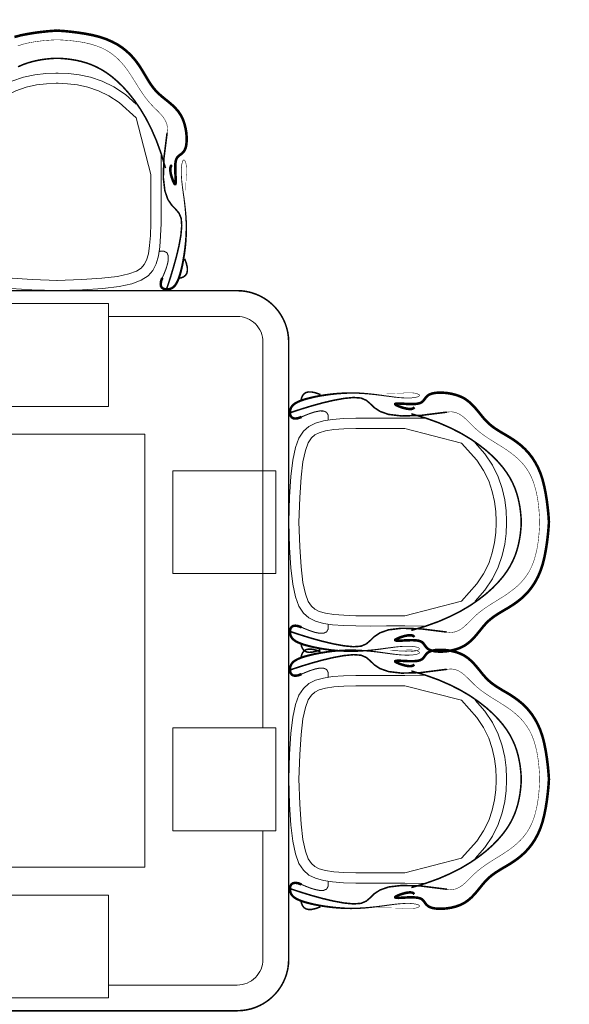
# Model space of a CAD drawing. Units: inches. Extents: x 513 to 1142, y 396 to 927.
# Tile 22 of 31: x 862 to 886, y 722 to 766. Entities that reach past the tile are written whole.
import ezdxf

# ---------------------------------------------------------------- set-up
doc = ezdxf.new("R2010")
doc.units = ezdxf.units.IN
doc.header["$MEASUREMENT"] = 0
doc.linetypes.add('DASHED', pattern=[0.75, 0.5, -0.25])
doc.layers.add('A-ANNO-DIMS', color=2, linetype='DASHED', lineweight=18)
doc.layers.add('furniture', color=92, linetype='Continuous', lineweight=18)
doc.styles.get("Standard").update_dxf_attribs({"font": 'arial.ttf'})
doc.dimstyles.get("Standard").update_dxf_attribs({"dimtxt": 4, "dimasz": 0.18, "dimexe": 0.18, "dimexo": 0.0625, "dimgap": 0.09, "dimtad": 0, "dimtih": 1, "dimtoh": 1, "dimdec": 0, "dimrnd": 6, "dimzin": 0, "dimdsep": 46, "dimlunit": 3, "dimtxsty": 'Standard', "dimcen": 0.09, "dimadec": 0, "dimazin": 0, "dimtfac": 1, "dimtdec": 0, "dimtofl": 0, "dimtmove": 0, "dimatfit": 3, "dimfxl": 1, "dimtolj": 1, "dimtzin": 0, "dimarcsym": 0})

# ---------------------------------------------------------------- blocks, each defined once
blk = doc.blocks.new('ОГ55_на6персон_стол1400х900')
at = {"const_width": 3}
blk.add_lwpolyline([(-600, 279.3), (600, 279.3, -0.414214), (700, 179.3), (700, -520.7, -0.414214), (600, -620.7), (-600, -620.7, -0.414214), (-700, -520.7), (-700, 179.3, -0.414214)], format="xyb", close=True, dxfattribs=at)
for points, const_width in [([(1193.2, -87.7), (1196.7, -101.2), (1199.4, -115.3), (1201.6, -129.2), (1203.2, -142.1), (1204.4, -153.5), (1205.1, -162.5), (1205.5, -168.5), (1205.7, -170.7)], 5), ([(1135.3, -94.9), (1139.6, -104.7), (1143, -114.3), (1145.6, -123.7), (1147.7, -132.7), (1149.2, -141.4), (1150.3, -149.3), (1151, -156.4), (1151.5, -162.3), (1151.7, -166.8), (1151.8, -169.6), (1151.8, -170.7)], 3), ([(1175.9, -94), (1179.3, -105.1), (1182.2, -117.4), (1184.5, -130.9), (1186.2, -145.8), (1187.4, -162.1), (1187.8, -170.7)], 1), ([(944.1, -394.1), (942.1, -391.9), (938.9, -390.8), (934.9, -390.6), (930.3, -391.1), (925.5, -392), (920.8, -393.4), (916.4, -394.9), (912.7, -396.3), (909.9, -397.6), (908, -398.7), (907.1, -399.6), (907.1, -400.3), (908, -400.8), (909.8, -401.1), (912.5, -401.2), (916.1, -401.2), (920.5, -401), (925.5, -400.7), (931, -400.4), (936.6, -400.2), (942.2, -400.3), (947.5, -400.6), (952.2, -401.3), (956.2, -402.5), (959.2, -404.2), (961.5, -406.4), (963.4, -408.8), (965.3, -411.4), (967.4, -414.1), (969.9, -416.5), (973.4, -418.7), (977.9, -420.5), (983.8, -421.8), (990.9, -422.4), (998.8, -422.4), (1007.3, -421.7), (1016.1, -420.3), (1024.9, -418), (1033.4, -415), (1041.3, -411), (1048.4, -406.2), (1054.8, -400.7), (1060.7, -394.6), (1066.3, -388.1), (1071.6, -381.6), (1076.9, -375), (1082.4, -368.7), (1088.1, -362.9), (1094.4, -357.6), (1101, -352.8), (1108, -348.2), (1115.2, -343.9), (1122.6, -339.5), (1130.1, -335), (1137.6, -330.2), (1145, -324.9), (1152.3, -319), (1159.4, -312.4), (1166.2, -305), (1172.7, -296.8), (1178.7, -287.6), (1184.1, -277.4), (1189, -266.1), (1193.2, -253.7), (1196.7, -240.1), (1199.4, -226.1), (1201.6, -212.2), (1203.2, -199.2), (1204.4, -187.9), (1205.1, -178.9), (1205.5, -172.9), (1205.7, -170.7)], 5), ([(938.3, -381.3), (966.1, -373), (991.4, -363.8), (1014.2, -353.9), (1034.8, -343.4), (1053.1, -332.5), (1069.4, -321.3), (1083.7, -310), (1096.1, -298.9), (1106.8, -287.9), (1116, -277.2), (1123.7, -266.7), (1130.1, -256.4), (1135.3, -246.4), (1139.6, -236.6), (1143, -227), (1145.6, -217.7), (1147.7, -208.6), (1149.2, -200), (1150.3, -192), (1151, -185), (1151.5, -179.1), (1151.7, -174.6), (1151.8, -171.7), (1151.8, -170.7)], 3), ([(1007.2, -384.5), (1015.9, -385.3), (1023.6, -384), (1030.7, -381.1), (1037.3, -376.9), (1043.5, -371.8), (1049.4, -366), (1055.3, -360), (1061.3, -354.1), (1067.5, -348.6), (1073.9, -343.4), (1080.6, -338.6), (1087.4, -334), (1094.3, -329.5), (1101.4, -325.1), (1108.5, -320.7), (1115.7, -316.1), (1122.9, -311.4), (1130, -306.5), (1137, -301.2), (1143.8, -295.4), (1150.3, -289.2), (1156.4, -282.3), (1162.1, -274.8), (1167.3, -266.5), (1171.9, -257.4), (1175.9, -247.3), (1179.3, -236.2), (1182.2, -224), (1184.5, -210.5), (1186.2, -195.6), (1187.4, -179.3), (1187.8, -170.7)], 1), ([(1007.2, -384.5), (956.2, -378.1), (919.4, -377.1), (894.1, -380.1), (877.3, -385.9), (866.4, -393.3), (858.5, -400.9), (850.8, -407.5), (840.7, -411.8), (826, -412.9), (807.4, -411.2), (786.6, -407.4), (765.2, -402.3), (744.5, -396.5), (726.1, -391), (711.6, -386.3), (702.6, -383.2)], 3), ([(724.9, -375.1), (732.7, -378.5), (741.6, -382), (751, -385), (760, -386.8), (767.8, -386.7), (773.6, -384.2), (776.8, -378.4), (776.4, -368.9)], 2), ([(761.7, -418.7), (752.5, -422), (744.8, -423.7), (738.5, -423.8), (733.5, -422.6), (729.7, -420.1), (726.9, -416.5), (725, -411.9), (723.8, -406.4)], 3), ([(-463.8, -927.9), (-457.4, -876.9), (-456.4, -840.1), (-459.4, -814.7), (-465.3, -798), (-472.6, -787), (-480.2, -779.2), (-486.8, -771.5), (-491.2, -761.4), (-492.3, -746.6), (-490.5, -728.1), (-486.7, -707.3), (-481.6, -685.8), (-475.9, -665.1), (-470.3, -646.8), (-465.6, -632.3), (-462.5, -623.2)], 3), ([(-36.2, -927.9), (-42.6, -876.9), (-43.6, -840.1), (-40.6, -814.7), (-34.7, -798), (-27.4, -787), (-19.8, -779.2), (-13.2, -771.5), (-8.8, -761.4), (-7.7, -746.6), (-9.5, -728.1), (-13.3, -707.3), (-18.4, -685.8), (-24.1, -665.1), (-29.7, -646.8), (-34.4, -632.3), (-37.5, -623.2)], 3), ([(36.2, -927.9), (42.6, -876.9), (43.6, -840.1), (40.6, -814.7), (34.7, -798), (27.4, -787), (19.8, -779.2), (13.2, -771.5), (8.8, -761.4), (7.7, -746.6), (9.5, -728.1), (13.3, -707.3), (18.4, -685.8), (24.1, -665.1), (29.7, -646.8), (34.4, -632.3), (37.5, -623.2)], 3), ([(463.8, -927.9), (457.4, -876.9), (456.4, -840.1), (459.4, -814.7), (465.3, -798), (472.6, -787), (480.2, -779.2), (486.8, -771.5), (491.2, -761.4), (492.3, -746.6), (490.5, -728.1), (486.7, -707.3), (481.6, -685.8), (475.9, -665.1), (470.3, -646.8), (465.6, -632.3), (462.5, -623.2)], 3), ([(-498, -682.4), (-501.3, -673.2), (-503, -665.5), (-503.1, -659.2), (-501.9, -654.2), (-499.4, -650.4), (-495.8, -647.6), (-491.2, -645.6), (-485.7, -644.5)], 3), ([(-454.5, -645.6), (-457.8, -653.4), (-461.3, -662.3), (-464.3, -671.7), (-466.1, -680.7), (-466, -688.5), (-463.5, -694.3), (-457.8, -697.5), (-448.2, -697.1)], 2), ([(-45.5, -645.6), (-42.2, -653.4), (-38.7, -662.3), (-35.7, -671.7), (-33.9, -680.7), (-34, -688.5), (-36.5, -694.3), (-42.2, -697.5), (-51.8, -697.1)], 2), ([(-2, -682.4), (1.3, -673.2), (3, -665.5), (3.1, -659.2), (1.9, -654.2), (-0.6, -650.4), (-4.2, -647.6), (-8.8, -645.6), (-14.3, -644.5)], 3), ([(2, -682.4), (-1.3, -673.2), (-3, -665.5), (-3.1, -659.2), (-1.9, -654.2), (0.6, -650.4), (4.2, -647.6), (8.8, -645.6), (14.3, -644.5)], 3), ([(45.5, -645.6), (42.2, -653.4), (38.7, -662.3), (35.7, -671.7), (33.9, -680.7), (34, -688.5), (36.5, -694.3), (42.2, -697.5), (51.8, -697.1)], 2), ([(454.5, -645.6), (457.8, -653.4), (461.3, -662.3), (464.3, -671.7), (466.1, -680.7), (466, -688.5), (463.5, -694.3), (457.8, -697.5), (448.2, -697.1)], 2), ([(498, -682.4), (501.3, -673.2), (503, -665.5), (503.1, -659.2), (501.9, -654.2), (499.4, -650.4), (495.8, -647.6), (491.2, -645.6), (485.7, -644.5)], 3), ([(-473.4, -864.8), (-471.2, -862.7), (-470.1, -859.6), (-469.9, -855.5), (-470.4, -851), (-471.4, -846.2), (-472.7, -841.5), (-474.2, -837.1), (-475.7, -833.4), (-477, -830.6), (-478, -828.7), (-478.9, -827.8), (-479.6, -827.7), (-480.1, -828.6), (-480.4, -830.5), (-480.6, -833.2), (-480.5, -836.7), (-480.3, -841.2), (-480, -846.2), (-479.7, -851.7), (-479.6, -857.3), (-479.6, -862.9), (-479.9, -868.2), (-480.6, -872.9), (-481.8, -876.8), (-483.5, -879.9), (-485.7, -882.2), (-488.2, -884.1), (-490.8, -886), (-493.4, -888), (-495.9, -890.6), (-498.1, -894), (-499.8, -898.6), (-501.1, -904.5), (-501.7, -911.6), (-501.7, -919.5), (-501, -928), (-499.6, -936.8), (-497.4, -945.6), (-494.3, -954.1), (-490.4, -962), (-485.5, -969.1), (-480, -975.5), (-473.9, -981.4), (-467.5, -986.9), (-460.9, -992.3), (-454.3, -997.6), (-448.1, -1003), (-442.2, -1008.8), (-436.9, -1015.1), (-432.1, -1021.7), (-427.6, -1028.7), (-423.2, -1035.9), (-418.9, -1043.3), (-414.4, -1050.8), (-409.5, -1058.3), (-404.2, -1065.7), (-398.3, -1073), (-391.7, -1080.1), (-384.3, -1086.9), (-376.1, -1093.3), (-366.9, -1099.3), (-356.7, -1104.8), (-345.4, -1109.7), (-333, -1113.9), (-319.5, -1117.3), (-305.4, -1120.1), (-291.5, -1122.3), (-278.6, -1123.9), (-267.2, -1125.1), (-258.2, -1125.8), (-252.2, -1126.2), (-250, -1126.3)], 5), ([(-26.6, -864.8), (-28.8, -862.7), (-29.9, -859.6), (-30.1, -855.5), (-29.6, -851), (-28.6, -846.2), (-27.3, -841.5), (-25.8, -837.1), (-24.3, -833.4), (-23, -830.6), (-22, -828.7), (-21.1, -827.8), (-20.4, -827.7), (-19.9, -828.6), (-19.6, -830.5), (-19.4, -833.2), (-19.5, -836.7), (-19.7, -841.2), (-20, -846.2), (-20.3, -851.7), (-20.4, -857.3), (-20.4, -862.9), (-20.1, -868.2), (-19.4, -872.9), (-18.2, -876.8), (-16.5, -879.9), (-14.3, -882.2), (-11.8, -884.1), (-9.2, -886), (-6.6, -888), (-4.1, -890.6), (-1.9, -894), (-0.2, -898.6), (1.1, -904.5), (1.7, -911.6), (1.7, -919.5), (1, -928), (-0.4, -936.8), (-2.6, -945.6), (-5.7, -954.1), (-9.6, -962), (-14.5, -969.1), (-20, -975.5), (-26.1, -981.4), (-32.5, -986.9), (-39.1, -992.3), (-45.7, -997.6), (-51.9, -1003), (-57.8, -1008.8), (-63.1, -1015.1), (-67.9, -1021.7), (-72.4, -1028.7), (-76.8, -1035.9), (-81.1, -1043.3), (-85.6, -1050.8), (-90.5, -1058.3), (-95.8, -1065.7), (-101.7, -1073), (-108.3, -1080.1), (-115.7, -1086.9), (-123.9, -1093.3), (-133.1, -1099.3), (-143.3, -1104.8), (-154.6, -1109.7), (-167, -1113.9), (-180.5, -1117.3), (-194.6, -1120.1), (-208.5, -1122.3), (-221.4, -1123.9), (-232.8, -1125.1), (-241.8, -1125.8), (-247.8, -1126.2), (-250, -1126.3)], 5), ([(26.6, -864.8), (28.8, -862.7), (29.9, -859.6), (30.1, -855.5), (29.6, -851), (28.6, -846.2), (27.3, -841.5), (25.8, -837.1), (24.3, -833.4), (23, -830.6), (22, -828.7), (21.1, -827.8), (20.4, -827.7), (19.9, -828.6), (19.6, -830.5), (19.4, -833.2), (19.5, -836.7), (19.7, -841.2), (20, -846.2), (20.3, -851.7), (20.4, -857.3), (20.4, -862.9), (20.1, -868.2), (19.4, -872.9), (18.2, -876.8), (16.5, -879.9), (14.3, -882.2), (11.8, -884.1), (9.2, -886), (6.6, -888), (4.1, -890.6), (1.9, -894), (0.2, -898.6), (-1.1, -904.5), (-1.7, -911.6), (-1.7, -919.5), (-1, -928), (0.4, -936.8), (2.6, -945.6), (5.7, -954.1), (9.6, -962), (14.5, -969.1), (20, -975.5), (26.1, -981.4), (32.5, -986.9), (39.1, -992.3), (45.7, -997.6), (51.9, -1003), (57.8, -1008.8), (63.1, -1015.1), (67.9, -1021.7), (72.4, -1028.7), (76.8, -1035.9), (81.1, -1043.3), (85.6, -1050.8), (90.5, -1058.3), (95.8, -1065.7), (101.7, -1073), (108.3, -1080.1), (115.7, -1086.9), (123.9, -1093.3), (133.1, -1099.3), (143.3, -1104.8), (154.6, -1109.7), (167, -1113.9), (180.5, -1117.3), (194.6, -1120.1), (208.5, -1122.3), (221.4, -1123.9), (232.8, -1125.1), (241.8, -1125.8), (247.8, -1126.2), (250, -1126.3)], 5), ([(473.4, -864.8), (471.2, -862.7), (470.1, -859.6), (469.9, -855.5), (470.4, -851), (471.4, -846.2), (472.7, -841.5), (474.2, -837.1), (475.7, -833.4), (477, -830.6), (478, -828.7), (478.9, -827.8), (479.6, -827.7), (480.1, -828.6), (480.4, -830.5), (480.6, -833.2), (480.5, -836.7), (480.3, -841.2), (480, -846.2), (479.7, -851.7), (479.6, -857.3), (479.6, -862.9), (479.9, -868.2), (480.6, -872.9), (481.8, -876.8), (483.5, -879.9), (485.7, -882.2), (488.2, -884.1), (490.8, -886), (493.4, -888), (495.9, -890.6), (498.1, -894), (499.8, -898.6), (501.1, -904.5), (501.7, -911.6), (501.7, -919.5), (501, -928), (499.6, -936.8), (497.4, -945.6), (494.3, -954.1), (490.4, -962), (485.5, -969.1), (480, -975.5), (473.9, -981.4), (467.5, -986.9), (460.9, -992.3), (454.3, -997.6), (448.1, -1003), (442.2, -1008.8), (436.9, -1015.1), (432.1, -1021.7), (427.6, -1028.7), (423.2, -1035.9), (418.9, -1043.3), (414.4, -1050.8), (409.5, -1058.3), (404.2, -1065.7), (398.3, -1073), (391.7, -1080.1), (384.3, -1086.9), (376.1, -1093.3), (366.9, -1099.3), (356.7, -1104.8), (345.4, -1109.7), (333, -1113.9), (319.5, -1117.3), (305.4, -1120.1), (291.5, -1122.3), (278.6, -1123.9), (267.2, -1125.1), (258.2, -1125.8), (252.2, -1126.2), (250, -1126.3)], 5), ([(-460.6, -859), (-452.3, -886.8), (-443.2, -912.1), (-433.2, -934.9), (-422.7, -955.5), (-411.8, -973.8), (-400.6, -990), (-389.4, -1004.3), (-378.2, -1016.8), (-367.2, -1027.5), (-356.5, -1036.7), (-346, -1044.4), (-335.8, -1050.8), (-325.7, -1056), (-315.9, -1060.3), (-306.4, -1063.6), (-297, -1066.3), (-287.9, -1068.3), (-279.3, -1069.9), (-271.3, -1071), (-264.3, -1071.7), (-258.4, -1072.2), (-253.9, -1072.4), (-251, -1072.5), (-250, -1072.5)], 3), ([(-39.4, -859), (-47.7, -886.8), (-56.8, -912.1), (-66.8, -934.9), (-77.3, -955.5), (-88.2, -973.8), (-99.4, -990), (-110.6, -1004.3), (-121.8, -1016.8), (-132.8, -1027.5), (-143.5, -1036.7), (-154, -1044.4), (-164.2, -1050.8), (-174.3, -1056), (-184.1, -1060.3), (-193.6, -1063.6), (-203, -1066.3), (-212.1, -1068.3), (-220.7, -1069.9), (-228.7, -1071), (-235.7, -1071.7), (-241.6, -1072.2), (-246.1, -1072.4), (-249, -1072.5), (-250, -1072.5)], 3), ([(39.4, -859), (47.7, -886.8), (56.8, -912.1), (66.8, -934.9), (77.3, -955.5), (88.2, -973.8), (99.4, -990), (110.6, -1004.3), (121.8, -1016.8), (132.8, -1027.5), (143.5, -1036.7), (154, -1044.4), (164.2, -1050.8), (174.3, -1056), (184.1, -1060.3), (193.6, -1063.6), (203, -1066.3), (212.1, -1068.3), (220.7, -1069.9), (228.7, -1071), (235.7, -1071.7), (241.6, -1072.2), (246.1, -1072.4), (249, -1072.5), (250, -1072.5)], 3), ([(460.6, -859), (452.3, -886.8), (443.2, -912.1), (433.2, -934.9), (422.7, -955.5), (411.8, -973.8), (400.6, -990), (389.4, -1004.3), (378.2, -1016.8), (367.2, -1027.5), (356.5, -1036.7), (346, -1044.4), (335.8, -1050.8), (325.7, -1056), (315.9, -1060.3), (306.4, -1063.6), (297, -1066.3), (287.9, -1068.3), (279.3, -1069.9), (271.3, -1071), (264.3, -1071.7), (258.4, -1072.2), (253.9, -1072.4), (251, -1072.5), (250, -1072.5)], 3), ([(-463.8, -927.9), (-464.6, -936.5), (-463.4, -944.3), (-460.5, -951.4), (-456.3, -958), (-451.1, -964.1), (-445.3, -970.1), (-439.3, -976), (-433.4, -982), (-427.9, -988.2), (-422.8, -994.6), (-417.9, -1001.3), (-413.3, -1008.1), (-408.8, -1015), (-404.4, -1022.1), (-400, -1029.2), (-395.5, -1036.4), (-390.8, -1043.6), (-385.8, -1050.7), (-380.5, -1057.7), (-374.7, -1064.5), (-368.5, -1071), (-361.7, -1077.1), (-354.1, -1082.8), (-345.9, -1088), (-336.7, -1092.6), (-326.7, -1096.6), (-315.5, -1100), (-303.3, -1102.9), (-289.8, -1105.2), (-274.9, -1106.9), (-258.6, -1108.1), (-250, -1108.4)], 1), ([(-36.2, -927.9), (-35.4, -936.5), (-36.6, -944.3), (-39.5, -951.4), (-43.7, -958), (-48.9, -964.1), (-54.7, -970.1), (-60.7, -976), (-66.6, -982), (-72.1, -988.2), (-77.2, -994.6), (-82.1, -1001.3), (-86.7, -1008.1), (-91.2, -1015), (-95.6, -1022.1), (-100, -1029.2), (-104.5, -1036.4), (-109.2, -1043.6), (-114.2, -1050.7), (-119.5, -1057.7), (-125.3, -1064.5), (-131.5, -1071), (-138.3, -1077.1), (-145.9, -1082.8), (-154.1, -1088), (-163.3, -1092.6), (-173.3, -1096.6), (-184.5, -1100), (-196.7, -1102.9), (-210.2, -1105.2), (-225.1, -1106.9), (-241.4, -1108.1), (-250, -1108.4)], 1), ([(36.2, -927.9), (35.4, -936.5), (36.6, -944.3), (39.5, -951.4), (43.7, -958), (48.9, -964.1), (54.7, -970.1), (60.7, -976), (66.6, -982), (72.1, -988.2), (77.2, -994.6), (82.1, -1001.3), (86.7, -1008.1), (91.2, -1015), (95.6, -1022.1), (100, -1029.2), (104.5, -1036.4), (109.2, -1043.6), (114.2, -1050.7), (119.5, -1057.7), (125.3, -1064.5), (131.5, -1071), (138.3, -1077.1), (145.9, -1082.8), (154.1, -1088), (163.3, -1092.6), (173.3, -1096.6), (184.5, -1100), (196.7, -1102.9), (210.2, -1105.2), (225.1, -1106.9), (241.4, -1108.1), (250, -1108.4)], 1), ([(463.8, -927.9), (464.6, -936.5), (463.4, -944.3), (460.5, -951.4), (456.3, -958), (451.1, -964.1), (445.3, -970.1), (439.3, -976), (433.4, -982), (427.9, -988.2), (422.8, -994.6), (417.9, -1001.3), (413.3, -1008.1), (408.8, -1015), (404.4, -1022.1), (400, -1029.2), (395.5, -1036.4), (390.8, -1043.6), (385.8, -1050.7), (380.5, -1057.7), (374.7, -1064.5), (368.5, -1071), (361.7, -1077.1), (354.1, -1082.8), (345.9, -1088), (336.7, -1092.6), (326.7, -1096.6), (315.5, -1100), (303.3, -1102.9), (289.8, -1105.2), (274.9, -1106.9), (258.6, -1108.1), (250, -1108.4)], 1)]:
    blk.add_lwpolyline(points, dxfattribs=dict(const_width=const_width))
for points in [[(966.1, 31.7), (925.8, 31.2), (889.9, 31.2), (858.2, 31.3), (830.4, 31.2), (806.3, 30.5), (785.4, 29), (767.4, 26.2), (752.2, 21.8), (739.4, 15.4), (728.7, 6.1), (720.1, -7.2), (713.2, -25.6), (708, -50.1), (704.2, -81.7), (701.6, -121.6), (700, -170.7)], [(1035.7, -17.1), (925.9, 11.2), (889.9, 11.2), (858.2, 11.3), (830.8, 11.2), (807.3, 10.5), (787.6, 9.1), (771.7, 6.6), (759.5, 3.1), (750.6, -1.3), (744, -7.1), (738, -16.3), (732.5, -31.2), (727.7, -53.4), (724.1, -83.6), (721.5, -122.5), (720, -171.3)], [(1035.7, -17.1), (1065.6, -50.4), (1078.8, -70.2), (1088.7, -90.5), (1095.5, -110.8), (1100, -130.9), (1102.3, -150.3), (1103.1, -168.6), (1103.1, -170.3)], [(1062.3, -16.7), (1081.4, -38.1), (1096.2, -60.3), (1107.2, -82.9), (1114.8, -105.5), (1119.7, -127.5), (1122.3, -148.6), (1123.1, -168.3), (1123.1, -170.7)], [(966.1, -373), (925.8, -372.6), (889.9, -372.6), (858.2, -372.7), (830.4, -372.6), (806.3, -371.9), (785.4, -370.3), (767.4, -367.5), (752.2, -363.2), (739.4, -356.8), (728.7, -347.5), (720.1, -334.1), (713.2, -315.8), (708, -291.3), (704.2, -259.6), (701.6, -219.8), (700, -170.7)], [(1035.7, -324.3), (925.9, -352.6), (889.9, -352.6), (858.2, -352.7), (830.8, -352.6), (807.3, -351.9), (787.6, -350.4), (771.7, -348), (759.5, -344.4), (750.6, -340), (744, -334.2), (738, -325.1), (732.5, -310.2), (727.7, -288), (724.1, -257.8), (721.5, -218.8), (720, -170)], [(1035.7, -324.3), (1065.6, -291), (1078.8, -271.1), (1088.7, -250.9), (1095.5, -230.5), (1100, -210.5), (1102.3, -191.1), (1103.1, -172.8), (1103.1, -171.1)], [(1062.3, -324.6), (1081.4, -303.3), (1096.2, -281.1), (1107.2, -258.5), (1114.8, -235.9), (1119.7, -213.8), (1122.3, -192.7), (1123.1, -173), (1123.1, -170.7)], [(-452.3, -886.8), (-451.9, -846.4), (-451.9, -810.6), (-452, -778.9), (-451.9, -751.1), (-451.2, -726.9), (-449.6, -706), (-446.8, -688.1), (-442.5, -672.9), (-436.1, -660), (-426.8, -649.4), (-413.5, -640.7), (-395.1, -633.9), (-370.6, -628.7), (-339, -624.8), (-299.1, -622.2), (-250, -620.7)], [(-47.7, -886.8), (-48.1, -846.4), (-48.1, -810.6), (-48, -778.9), (-48.1, -751.1), (-48.8, -726.9), (-50.4, -706), (-53.2, -688.1), (-57.5, -672.9), (-63.9, -660), (-73.2, -649.4), (-86.5, -640.7), (-104.9, -633.9), (-129.4, -628.7), (-161, -624.8), (-200.9, -622.2), (-250, -620.7)], [(47.7, -886.8), (48.1, -846.4), (48.1, -810.6), (48, -778.9), (48.1, -751.1), (48.8, -726.9), (50.4, -706), (53.2, -688.1), (57.5, -672.9), (63.9, -660), (73.2, -649.4), (86.5, -640.7), (104.9, -633.9), (129.4, -628.7), (161, -624.8), (200.9, -622.2), (250, -620.7)], [(452.3, -886.8), (451.9, -846.4), (451.9, -810.6), (452, -778.9), (451.9, -751.1), (451.2, -726.9), (449.6, -706), (446.8, -688.1), (442.5, -672.9), (436.1, -660), (426.8, -649.4), (413.5, -640.7), (395.1, -633.9), (370.6, -628.7), (339, -624.8), (299.1, -622.2), (250, -620.7)], [(-403.6, -956.4), (-431.9, -846.6), (-431.9, -810.5), (-432, -778.9), (-431.9, -751.4), (-431.2, -728), (-429.8, -708.3), (-427.3, -692.4), (-423.8, -680.1), (-419.4, -671.3), (-413.6, -664.7), (-404.4, -658.7), (-389.5, -653.1), (-367.3, -648.4), (-337.1, -644.8), (-298.1, -642.2), (-249.4, -640.7)], [(-96.4, -956.4), (-68.1, -846.6), (-68.1, -810.5), (-68, -778.9), (-68.1, -751.4), (-68.8, -728), (-70.2, -708.3), (-72.7, -692.4), (-76.2, -680.1), (-80.6, -671.3), (-86.4, -664.7), (-95.6, -658.7), (-110.5, -653.1), (-132.7, -648.4), (-162.9, -644.8), (-201.9, -642.2), (-250.6, -640.7)], [(96.4, -956.4), (68.1, -846.6), (68.1, -810.5), (68, -778.9), (68.1, -751.4), (68.8, -728), (70.2, -708.3), (72.7, -692.4), (76.2, -680.1), (80.6, -671.3), (86.4, -664.7), (95.6, -658.7), (110.5, -653.1), (132.7, -648.4), (162.9, -644.8), (201.9, -642.2), (250.6, -640.7)], [(403.6, -956.4), (431.9, -846.6), (431.9, -810.5), (432, -778.9), (431.9, -751.4), (431.2, -728), (429.8, -708.3), (427.3, -692.4), (423.8, -680.1), (419.4, -671.3), (413.6, -664.7), (404.4, -658.7), (389.5, -653.1), (367.3, -648.4), (337.1, -644.8), (298.1, -642.2), (249.4, -640.7)], [(-403.6, -956.4), (-370.3, -986.3), (-350.5, -999.5), (-330.2, -1009.3), (-309.8, -1016.2), (-289.8, -1020.6), (-270.4, -1023), (-252.1, -1023.8), (-250.4, -1023.8)], [(-96.4, -956.4), (-129.7, -986.3), (-149.5, -999.5), (-169.8, -1009.3), (-190.2, -1016.2), (-210.2, -1020.6), (-229.6, -1023), (-247.9, -1023.8), (-249.6, -1023.8)], [(96.4, -956.4), (129.7, -986.3), (149.5, -999.5), (169.8, -1009.3), (190.2, -1016.2), (210.2, -1020.6), (229.6, -1023), (247.9, -1023.8), (249.6, -1023.8)], [(403.6, -956.4), (370.3, -986.3), (350.5, -999.5), (330.2, -1009.3), (309.8, -1016.2), (289.8, -1020.6), (270.4, -1023), (252.1, -1023.8), (250.4, -1023.8)], [(-404, -983), (-382.6, -1002.1), (-360.4, -1016.9), (-337.8, -1027.9), (-315.2, -1035.5), (-293.1, -1040.4), (-272, -1043), (-252.3, -1043.8), (-250, -1043.8)], [(-96, -983), (-117.4, -1002.1), (-139.6, -1016.9), (-162.2, -1027.9), (-184.8, -1035.5), (-206.9, -1040.4), (-228, -1043), (-247.7, -1043.8), (-250, -1043.8)], [(96, -983), (117.4, -1002.1), (139.6, -1016.9), (162.2, -1027.9), (184.8, -1035.5), (206.9, -1040.4), (228, -1043), (247.7, -1043.8), (250, -1043.8)], [(404, -983), (382.6, -1002.1), (360.4, -1016.9), (337.8, -1027.9), (315.2, -1035.5), (293.1, -1040.4), (272, -1043), (252.3, -1043.8), (250, -1043.8)]]:
    blk.add_lwpolyline(points)
for points in [[(-420.7, -341.4), (420.7, -341.4), (420.7, 0), (-420.7, 0)], [(-675, -270.7), (-475, -270.7), (-475, -70.7), (-675, -70.7)], [(675, -270.7), (475, -270.7), (475, -70.7), (675, -70.7)], [(-150, -595.7), (-150, -395.7), (-350, -395.7), (-350, -595.7)], [(150, -595.7), (150, -395.7), (350, -395.7), (350, -595.7)]]:
    blk.add_lwpolyline(points, close=True)
for points, format in [([(-350, -570.7), (-600, -570.7, -0.414214), (-650, -520.7), (-650, -270.7)], "xyb"), ([(650, -270.7), (650, -520.7, -0.414214), (600, -570.7), (-150, -570.7)], "xyb"), ([(724.9, -375.1, 5, 4.91, 0), (718.1, -372.7, 4.91, 4.84, 0), (712.8, -372, 4.84, 4.78, 0), (708.7, -372.6, 4.78, 4.74, 0), (705.8, -374.3, 4.74, 4.7, 0), (703.9, -376.9, 4.7, 4.65, 0), (702.9, -380.1, 4.65, 4.61, 0), (702.5, -383.6, 4.61, 4.56, 0), (702.8, -387.1, 4.56, 4.52, 0), (703.5, -390.5, 4.52, 4.47, 0), (704.8, -393.6, 4.47, 4.43, 0), (706.7, -396.6, 4.43, 4.38, 0), (709.5, -399.3, 4.38, 4.32, 0), (713.2, -402, 4.32, 4.25, 0), (717.9, -404.5, 4.25, 4.17, 0), (723.8, -407, 4.17, 4.07, 0), (731, -409.4, 4.07, 3.95, 0), (739.6, -411.7, 3.95, 3.82, 0), (749.3, -414, 3.82, 3.68, 0), (760.1, -416, 3.68, 3.53, 0), (771.6, -417.9, 3.53, 3.37, 0), (783.7, -419.5, 3.37, 3.21, 0), (796.2, -420.7, 3.21, 3.05, 0), (808.8, -421.5, 3.05, 2.88, 0), (821.4, -421.8, 2.88, 2.72, 0), (833.8, -421.6, 2.72, 2.57, 0), (845.8, -420.9, 2.57, 2.41, 0), (857.4, -419.9, 2.41, 2.27, 0), (868.5, -418.7, 2.27, 2.13, 0), (879, -417.4, 2.13, 2, 0), (888.9, -416, 2, 1.88, 0), (898, -414.7, 1.88, 1.78, 0), (906.3, -413.7, 1.78, 1.68, 0), (913.7, -412.9, 1.68, 1.59, 0), (920.3, -412.4, 1.59, 1.52, 0), (926.1, -412.1, 1.52, 1.45, 0), (931.2, -412, 1.45, 1.4, 0), (935.6, -412.1, 1.4, 1.35, 0), (939.4, -412.3, 1.35, 1.3, 0), (942.6, -412.7, 1.3, 1.27, 0), (945.3, -413, 1.27, 1.24, 0), (947.6, -413.5, 1.24, 1.21, 0), (949.5, -413.9, 1.21, 1.19, 0), (951, -414.4, 1.19, 1.18, 0), (952.2, -414.9, 1.18, 1.16, 0), (953, -415.4, 1.16, 1.15, 0), (953.6, -416, 1.15, 1.14, 0), (953.9, -416.5, 1.14, 1.14, 0), (954, -417, 1.14, 1.13, 0), (953.9, -417.5, 1.13, 1.12, 0), (953.6, -418, 1.12, 1.12, 0), (953.2, -418.5, 1.12, 1.11, 0), (952.6, -418.9, 1.11, 1.09, 0), (951.8, -419.4, 1.09, 1.08, 0), (950.9, -419.8, 1.08, 1.07, 0), (949.8, -420.2, 1.07, 1.05, 0), (948.6, -420.6, 1.05, 1.03, 0), (947.2, -421, 1.03, 1.01, 0), (945.6, -421.3, 1.01, 0.986, 0), (943.8, -421.6, 0.986, 0.959, 0), (941.7, -421.8, 0.959, 0.926, 0), (939.2, -422, 0.926, 0.889, 0), (936.3, -422, 0.889, 0.846, 0), (933, -422, 0.846, 0.796, 0), (929.1, -422, 0.796, 0.738, 0), (924.7, -421.8, 0.738, 0.672, 0), (919.6, -421.5, 0.672, 0.595, 0), (913.7, -421.2, 0.595, 0.506, 0), (906.8, -421, 0.506, 0.404, 0), (898.9, -420.7, 0.404, 0.286, 0), (889.9, -420.6, 0.286, 0.152, 0), (879.5, -420.6, 0.152, 0, 0), (867.8, -420.7, 0, 0, 0)], "xyseb"), ([(-454.5, -645.6, 5, 4.91, 0), (-452, -638.8, 4.91, 4.84, 0), (-451.3, -633.5, 4.84, 4.78, 0), (-451.9, -629.4, 4.78, 4.74, 0), (-453.7, -626.5, 4.74, 4.7, 0), (-456.3, -624.6, 4.7, 4.65, 0), (-459.4, -623.5, 4.65, 4.61, 0), (-462.9, -623.2, 4.61, 4.56, 0), (-466.5, -623.5, 4.56, 4.52, 0), (-469.8, -624.2, 4.52, 4.47, 0), (-472.9, -625.5, 4.47, 4.43, 0), (-475.9, -627.4, 4.43, 4.38, 0), (-478.7, -630.2, 4.38, 4.32, 0), (-481.3, -633.9, 4.32, 4.25, 0), (-483.8, -638.6, 4.25, 4.17, 0), (-486.3, -644.5, 4.17, 4.07, 0), (-488.7, -651.7, 4.07, 3.95, 0), (-491, -660.3, 3.95, 3.82, 0), (-493.3, -670, 3.82, 3.68, 0), (-495.4, -680.8, 3.68, 3.53, 0), (-497.2, -692.3, 3.53, 3.37, 0), (-498.8, -704.4, 3.37, 3.21, 0), (-500, -716.9, 3.21, 3.05, 0), (-500.8, -729.5, 3.05, 2.88, 0), (-501.1, -742.1, 2.88, 2.72, 0), (-500.9, -754.5, 2.72, 2.57, 0), (-500.2, -766.5, 2.57, 2.41, 0), (-499.2, -778.1, 2.41, 2.27, 0), (-498, -789.2, 2.27, 2.13, 0), (-496.7, -799.7, 2.13, 2, 0), (-495.3, -809.6, 2, 1.88, 0), (-494.1, -818.7, 1.88, 1.78, 0), (-493, -827, 1.78, 1.68, 0), (-492.2, -834.4, 1.68, 1.59, 0), (-491.7, -841, 1.59, 1.52, 0), (-491.4, -846.8, 1.52, 1.45, 0), (-491.3, -851.9, 1.45, 1.4, 0), (-491.4, -856.3, 1.4, 1.35, 0), (-491.6, -860.1, 1.35, 1.3, 0), (-492, -863.3, 1.3, 1.27, 0), (-492.4, -866, 1.27, 1.24, 0), (-492.8, -868.3, 1.24, 1.21, 0), (-493.3, -870.2, 1.21, 1.19, 0), (-493.8, -871.7, 1.19, 1.18, 0), (-494.3, -872.9, 1.18, 1.16, 0), (-494.8, -873.7, 1.16, 1.15, 0), (-495.3, -874.3, 1.15, 1.14, 0), (-495.8, -874.6, 1.14, 1.14, 0), (-496.3, -874.7, 1.14, 1.13, 0), (-496.8, -874.6, 1.13, 1.12, 0), (-497.3, -874.3, 1.12, 1.12, 0), (-497.8, -873.9, 1.12, 1.11, 0), (-498.3, -873.3, 1.11, 1.09, 0), (-498.7, -872.5, 1.09, 1.08, 0), (-499.1, -871.6, 1.08, 1.07, 0), (-499.5, -870.5, 1.07, 1.05, 0), (-499.9, -869.2, 1.05, 1.03, 0), (-500.3, -867.9, 1.03, 1.01, 0), (-500.6, -866.3, 1.01, 0.986, 0), (-500.9, -864.5, 0.986, 0.959, 0), (-501.1, -862.4, 0.959, 0.926, 0), (-501.3, -859.9, 0.926, 0.889, 0), (-501.4, -857, 0.889, 0.846, 0), (-501.4, -853.7, 0.846, 0.796, 0), (-501.3, -849.8, 0.796, 0.738, 0), (-501.1, -845.4, 0.738, 0.672, 0), (-500.8, -840.3, 0.672, 0.595, 0), (-500.6, -834.3, 0.595, 0.506, 0), (-500.3, -827.5, 0.506, 0.404, 0), (-500.1, -819.6, 0.404, 0.286, 0), (-499.9, -810.5, 0.286, 0.152, 0), (-499.9, -800.2, 0.152, 0, 0), (-500, -788.5, 0, 0, 0)], "xyseb"), ([(-45.5, -645.6, 5, 4.91, 0), (-48, -638.8, 4.91, 4.84, 0), (-48.7, -633.5, 4.84, 4.78, 0), (-48.1, -629.4, 4.78, 4.74, 0), (-46.3, -626.5, 4.74, 4.7, 0), (-43.7, -624.6, 4.7, 4.65, 0), (-40.6, -623.5, 4.65, 4.61, 0), (-37.1, -623.2, 4.61, 4.56, 0), (-33.5, -623.5, 4.56, 4.52, 0), (-30.2, -624.2, 4.52, 4.47, 0), (-27.1, -625.5, 4.47, 4.43, 0), (-24.1, -627.4, 4.43, 4.38, 0), (-21.3, -630.2, 4.38, 4.32, 0), (-18.7, -633.9, 4.32, 4.25, 0), (-16.2, -638.6, 4.25, 4.17, 0), (-13.7, -644.5, 4.17, 4.07, 0), (-11.3, -651.7, 4.07, 3.95, 0), (-9, -660.3, 3.95, 3.82, 0), (-6.7, -670, 3.82, 3.68, 0), (-4.6, -680.8, 3.68, 3.53, 0), (-2.8, -692.3, 3.53, 3.37, 0), (-1.2, -704.4, 3.37, 3.21, 0), (0, -716.9, 3.21, 3.05, 0), (0.8, -729.5, 3.05, 2.88, 0), (1.1, -742.1, 2.88, 2.72, 0), (0.9, -754.5, 2.72, 2.57, 0), (0.2, -766.5, 2.57, 2.41, 0), (-0.8, -778.1, 2.41, 2.27, 0), (-2, -789.2, 2.27, 2.13, 0), (-3.3, -799.7, 2.13, 2, 0), (-4.7, -809.6, 2, 1.88, 0), (-5.9, -818.7, 1.88, 1.78, 0), (-7, -827, 1.78, 1.68, 0), (-7.8, -834.4, 1.68, 1.59, 0), (-8.3, -841, 1.59, 1.52, 0), (-8.6, -846.8, 1.52, 1.45, 0), (-8.7, -851.9, 1.45, 1.4, 0), (-8.6, -856.3, 1.4, 1.35, 0), (-8.4, -860.1, 1.35, 1.3, 0), (-8, -863.3, 1.3, 1.27, 0), (-7.6, -866, 1.27, 1.24, 0), (-7.2, -868.3, 1.24, 1.21, 0), (-6.7, -870.2, 1.21, 1.19, 0), (-6.2, -871.7, 1.19, 1.18, 0), (-5.7, -872.9, 1.18, 1.16, 0), (-5.2, -873.7, 1.16, 1.15, 0), (-4.7, -874.3, 1.15, 1.14, 0), (-4.2, -874.6, 1.14, 1.14, 0), (-3.7, -874.7, 1.14, 1.13, 0), (-3.2, -874.6, 1.13, 1.12, 0), (-2.7, -874.3, 1.12, 1.12, 0), (-2.2, -873.9, 1.12, 1.11, 0), (-1.7, -873.3, 1.11, 1.09, 0), (-1.3, -872.5, 1.09, 1.08, 0), (-0.9, -871.6, 1.08, 1.07, 0), (-0.5, -870.5, 1.07, 1.05, 0), (-0.1, -869.2, 1.05, 1.03, 0), (0.3, -867.9, 1.03, 1.01, 0), (0.6, -866.3, 1.01, 0.986, 0), (0.9, -864.5, 0.986, 0.959, 0), (1.1, -862.4, 0.959, 0.926, 0), (1.3, -859.9, 0.926, 0.889, 0), (1.4, -857, 0.889, 0.846, 0), (1.4, -853.7, 0.846, 0.796, 0), (1.3, -849.8, 0.796, 0.738, 0), (1.1, -845.4, 0.738, 0.672, 0), (0.8, -840.3, 0.672, 0.595, 0), (0.6, -834.3, 0.595, 0.506, 0), (0.3, -827.5, 0.506, 0.404, 0), (0.1, -819.6, 0.404, 0.286, 0), (-0.1, -810.5, 0.286, 0.152, 0), (-0.1, -800.2, 0.152, 0, 0), (0, -788.5, 0, 0, 0)], "xyseb"), ([(45.5, -645.6, 5, 4.91, 0), (48, -638.8, 4.91, 4.84, 0), (48.7, -633.5, 4.84, 4.78, 0), (48.1, -629.4, 4.78, 4.74, 0), (46.3, -626.5, 4.74, 4.7, 0), (43.7, -624.6, 4.7, 4.65, 0), (40.6, -623.5, 4.65, 4.61, 0), (37.1, -623.2, 4.61, 4.56, 0), (33.5, -623.5, 4.56, 4.52, 0), (30.2, -624.2, 4.52, 4.47, 0), (27.1, -625.5, 4.47, 4.43, 0), (24.1, -627.4, 4.43, 4.38, 0), (21.3, -630.2, 4.38, 4.32, 0), (18.7, -633.9, 4.32, 4.25, 0), (16.2, -638.6, 4.25, 4.17, 0), (13.7, -644.5, 4.17, 4.07, 0), (11.3, -651.7, 4.07, 3.95, 0), (9, -660.3, 3.95, 3.82, 0), (6.7, -670, 3.82, 3.68, 0), (4.6, -680.8, 3.68, 3.53, 0), (2.8, -692.3, 3.53, 3.37, 0), (1.2, -704.4, 3.37, 3.21, 0), (0, -716.9, 3.21, 3.05, 0), (-0.8, -729.5, 3.05, 2.88, 0), (-1.1, -742.1, 2.88, 2.72, 0), (-0.9, -754.5, 2.72, 2.57, 0), (-0.2, -766.5, 2.57, 2.41, 0), (0.8, -778.1, 2.41, 2.27, 0), (2, -789.2, 2.27, 2.13, 0), (3.3, -799.7, 2.13, 2, 0), (4.7, -809.6, 2, 1.88, 0), (5.9, -818.7, 1.88, 1.78, 0), (7, -827, 1.78, 1.68, 0), (7.8, -834.4, 1.68, 1.59, 0), (8.3, -841, 1.59, 1.52, 0), (8.6, -846.8, 1.52, 1.45, 0), (8.7, -851.9, 1.45, 1.4, 0), (8.6, -856.3, 1.4, 1.35, 0), (8.4, -860.1, 1.35, 1.3, 0), (8, -863.3, 1.3, 1.27, 0), (7.6, -866, 1.27, 1.24, 0), (7.2, -868.3, 1.24, 1.21, 0), (6.7, -870.2, 1.21, 1.19, 0), (6.2, -871.7, 1.19, 1.18, 0), (5.7, -872.9, 1.18, 1.16, 0), (5.2, -873.7, 1.16, 1.15, 0), (4.7, -874.3, 1.15, 1.14, 0), (4.2, -874.6, 1.14, 1.14, 0), (3.7, -874.7, 1.14, 1.13, 0), (3.2, -874.6, 1.13, 1.12, 0), (2.7, -874.3, 1.12, 1.12, 0), (2.2, -873.9, 1.12, 1.11, 0), (1.7, -873.3, 1.11, 1.09, 0), (1.3, -872.5, 1.09, 1.08, 0), (0.9, -871.6, 1.08, 1.07, 0), (0.5, -870.5, 1.07, 1.05, 0), (0.1, -869.2, 1.05, 1.03, 0), (-0.3, -867.9, 1.03, 1.01, 0), (-0.6, -866.3, 1.01, 0.986, 0), (-0.9, -864.5, 0.986, 0.959, 0), (-1.1, -862.4, 0.959, 0.926, 0), (-1.3, -859.9, 0.926, 0.889, 0), (-1.4, -857, 0.889, 0.846, 0), (-1.4, -853.7, 0.846, 0.796, 0), (-1.3, -849.8, 0.796, 0.738, 0), (-1.1, -845.4, 0.738, 0.672, 0), (-0.8, -840.3, 0.672, 0.595, 0), (-0.6, -834.3, 0.595, 0.506, 0), (-0.3, -827.5, 0.506, 0.404, 0), (-0.1, -819.6, 0.404, 0.286, 0), (0.1, -810.5, 0.286, 0.152, 0), (0.1, -800.2, 0.152, 0, 0), (0, -788.5, 0, 0, 0)], "xyseb"), ([(454.5, -645.6, 5, 4.91, 0), (452, -638.8, 4.91, 4.84, 0), (451.3, -633.5, 4.84, 4.78, 0), (451.9, -629.4, 4.78, 4.74, 0), (453.7, -626.5, 4.74, 4.7, 0), (456.3, -624.6, 4.7, 4.65, 0), (459.4, -623.5, 4.65, 4.61, 0), (462.9, -623.2, 4.61, 4.56, 0), (466.5, -623.5, 4.56, 4.52, 0), (469.8, -624.2, 4.52, 4.47, 0), (472.9, -625.5, 4.47, 4.43, 0), (475.9, -627.4, 4.43, 4.38, 0), (478.7, -630.2, 4.38, 4.32, 0), (481.3, -633.9, 4.32, 4.25, 0), (483.8, -638.6, 4.25, 4.17, 0), (486.3, -644.5, 4.17, 4.07, 0), (488.7, -651.7, 4.07, 3.95, 0), (491, -660.3, 3.95, 3.82, 0), (493.3, -670, 3.82, 3.68, 0), (495.4, -680.8, 3.68, 3.53, 0), (497.2, -692.3, 3.53, 3.37, 0), (498.8, -704.4, 3.37, 3.21, 0), (500, -716.9, 3.21, 3.05, 0), (500.8, -729.5, 3.05, 2.88, 0), (501.1, -742.1, 2.88, 2.72, 0), (500.9, -754.5, 2.72, 2.57, 0), (500.2, -766.5, 2.57, 2.41, 0), (499.2, -778.1, 2.41, 2.27, 0), (498, -789.2, 2.27, 2.13, 0), (496.7, -799.7, 2.13, 2, 0), (495.3, -809.6, 2, 1.88, 0), (494.1, -818.7, 1.88, 1.78, 0), (493, -827, 1.78, 1.68, 0), (492.2, -834.4, 1.68, 1.59, 0), (491.7, -841, 1.59, 1.52, 0), (491.4, -846.8, 1.52, 1.45, 0), (491.3, -851.9, 1.45, 1.4, 0), (491.4, -856.3, 1.4, 1.35, 0), (491.6, -860.1, 1.35, 1.3, 0), (492, -863.3, 1.3, 1.27, 0), (492.4, -866, 1.27, 1.24, 0), (492.8, -868.3, 1.24, 1.21, 0), (493.3, -870.2, 1.21, 1.19, 0), (493.8, -871.7, 1.19, 1.18, 0), (494.3, -872.9, 1.18, 1.16, 0), (494.8, -873.7, 1.16, 1.15, 0), (495.3, -874.3, 1.15, 1.14, 0), (495.8, -874.6, 1.14, 1.14, 0), (496.3, -874.7, 1.14, 1.13, 0), (496.8, -874.6, 1.13, 1.12, 0), (497.3, -874.3, 1.12, 1.12, 0), (497.8, -873.9, 1.12, 1.11, 0), (498.3, -873.3, 1.11, 1.09, 0), (498.7, -872.5, 1.09, 1.08, 0), (499.1, -871.6, 1.08, 1.07, 0), (499.5, -870.5, 1.07, 1.05, 0), (499.9, -869.2, 1.05, 1.03, 0), (500.3, -867.9, 1.03, 1.01, 0), (500.6, -866.3, 1.01, 0.986, 0), (500.9, -864.5, 0.986, 0.959, 0), (501.1, -862.4, 0.959, 0.926, 0), (501.3, -859.9, 0.926, 0.889, 0), (501.4, -857, 0.889, 0.846, 0), (501.4, -853.7, 0.846, 0.796, 0), (501.3, -849.8, 0.796, 0.738, 0), (501.1, -845.4, 0.738, 0.672, 0), (500.8, -840.3, 0.672, 0.595, 0), (500.6, -834.3, 0.595, 0.506, 0), (500.3, -827.5, 0.506, 0.404, 0), (500.1, -819.6, 0.404, 0.286, 0), (499.9, -810.5, 0.286, 0.152, 0), (499.9, -800.2, 0.152, 0, 0), (500, -788.5, 0, 0, 0)], "xyseb")]:
    blk.add_lwpolyline(points, format=format)
blk = doc.blocks.new('*D137')
at = {"layer": 'A-ANNO-DIMS', "color": 0, "lineweight": -2, "transparency": 16777216}
for p, q in [((839.995, 770.096), (839.995, 401.578)), ((920.995, 770.067), (920.995, 401.578)), ((840.175, 401.758), (875.078, 401.758)), ((920.815, 401.758), (885.913, 401.758))]:
    blk.add_line(p, q, dxfattribs=at)
at = {"layer": 'A-ANNO-DIMS', "color": 0, "transparency": 16777216}
for points in [[(840.175, 401.788), (840.175, 401.728), (839.995, 401.758)], [(920.815, 401.788), (920.815, 401.728), (920.995, 401.758)]]:
    blk.add_solid(points, dxfattribs=at)
at = {"layer": 'Defpoints', "color": 0, "transparency": 16777216}
for p in [(839.995, 770.158), (920.995, 770.13), (920.995, 401.758)]:
    blk.add_point(p, dxfattribs=at)
at = {"layer": 'A-ANNO-DIMS', "color": 0, "transparency": 16777216, "insert": (880.495, 401.758), "char_height": 4, "attachment_point": 5}
blk.add_mtext('\\A1;6\'-9"', dxfattribs=at)
blk = doc.blocks.new('*D149')
at = {"layer": 'A-ANNO-DIMS', "color": 0, "lineweight": -2, "transparency": 16777216}
for p, q in [((840.058, 770.158), (1131.575, 770.158)), ((1131.395, 769.978), (1131.395, 707.791)), ((1131.395, 641.338), (1131.395, 703.526)), ((840.058, 641.158), (1131.575, 641.158))]:
    blk.add_line(p, q, dxfattribs=at)
at = {"layer": 'A-ANNO-DIMS', "color": 0, "transparency": 16777216}
for points in [[(1131.365, 769.978), (1131.425, 769.978), (1131.395, 770.158)], [(1131.365, 641.338), (1131.425, 641.338), (1131.395, 641.158)]]:
    blk.add_solid(points, dxfattribs=at)
at = {"layer": 'Defpoints', "color": 0, "transparency": 16777216}
for p in [(839.995, 770.158), (1131.395, 770.158), (839.995, 641.158)]:
    blk.add_point(p, dxfattribs=at)
at = {"layer": 'A-ANNO-DIMS', "color": 0, "transparency": 16777216, "insert": (1131.395, 705.658), "char_height": 4, "attachment_point": 5}
blk.add_mtext('\\A1;10\'-9"', dxfattribs=at)
blk = doc.blocks.new('*D176')
at = {"layer": 'A-ANNO-DIMS', "color": 0, "lineweight": -2, "transparency": 16777216}
for p, q in [((847.995, 637.221), (847.995, 920.738)), ((891.995, 637.221), (891.995, 920.738)), ((848.175, 920.558), (864.59, 920.558)), ((891.815, 920.558), (875.4, 920.558))]:
    blk.add_line(p, q, dxfattribs=at)
at = {"layer": 'A-ANNO-DIMS', "color": 0, "transparency": 16777216}
for points in [[(848.175, 920.588), (848.175, 920.528), (847.995, 920.558)], [(891.815, 920.588), (891.815, 920.528), (891.995, 920.558)]]:
    blk.add_solid(points, dxfattribs=at)
at = {"layer": 'Defpoints', "color": 0, "transparency": 16777216}
for p in [(891.995, 920.558), (847.995, 637.158), (891.995, 637.158)]:
    blk.add_point(p, dxfattribs=at)
at = {"layer": 'A-ANNO-DIMS', "color": 0, "transparency": 16777216, "insert": (869.995, 920.558), "char_height": 4, "attachment_point": 5}
blk.add_mtext('\\A1;3\'-8"', dxfattribs=at)

msp = doc.modelspace()

# ---------------------------------------------------------------- block references
at = {"layer": 'furniture', "xscale": 0.022676467704094, "yscale": 0.022676467704094, "zscale": 0.022676467704094, "rotation": 90}
msp.add_blockref('ОГ55_на6персон_стол1400х900', (859.781, 737.859), dxfattribs=at)

# ---------------------------------------------------------------- dimensions: what is measured, and where the dimension line sits
at = {"layer": 'A-ANNO-DIMS'}
for base, p1, p2, picture, middle in [((891.995, 920.558), (847.995, 637.158), (891.995, 637.158), '*D176', (869.995, 920.558)), ((920.995, 401.758), (839.995, 770.158), (920.995, 770.13), '*D137', (880.495, 401.758))]:
    dim = msp.add_linear_dim(base=base, p1=p1, p2=p2, dimstyle='Standard', override={"dimdec": 1, "dimlfac": 1, "dimrnd": 0, "dimzin": 1, "dimdsep": 46, "dimlunit": 4, "dimfrac": 2}, dxfattribs=at)
    dim.commit()
    dim.dimension.update_dxf_attribs({"geometry": picture, "text_midpoint": middle})
dim = msp.add_linear_dim(base=(1131.395, 770.158), p1=(839.995, 641.158), p2=(839.995, 770.158), angle=90, dimstyle='Standard', override={"dimdec": 1, "dimlfac": 1, "dimrnd": 0, "dimzin": 1, "dimdsep": 46, "dimlunit": 4, "dimfrac": 2}, dxfattribs=at)
dim.commit()
dim.dimension.update_dxf_attribs({"geometry": '*D149', "text_midpoint": (1131.395, 705.658)})

doc.saveas('drawing.dxf')
